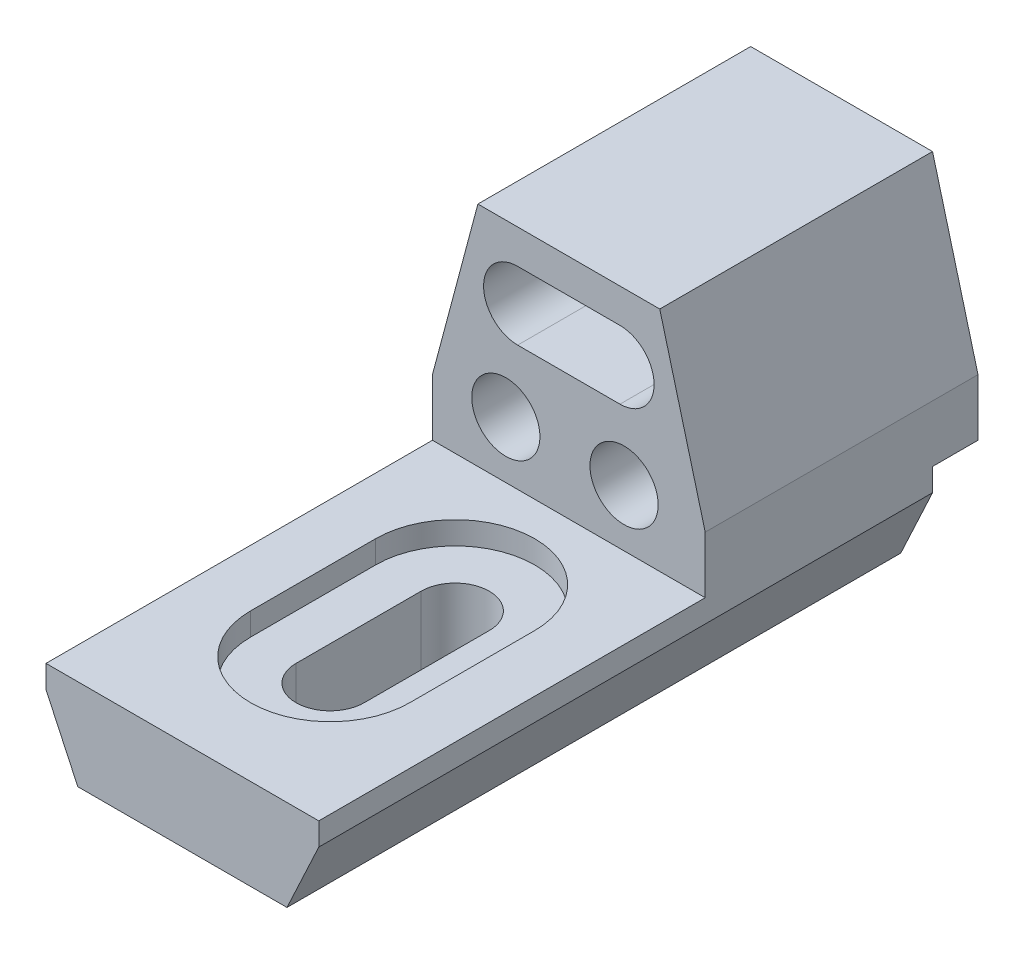
ISO-10303-21;
HEADER;
FILE_DESCRIPTION(('STEP AP214'),'2;1');
FILE_NAME('part.step','',(''),(''),'','','');
FILE_SCHEMA(('AUTOMOTIVE_DESIGN { 1 0 10303 214 1 1 1 1 }'));
ENDSEC;
DATA;
#1=APPLICATION_CONTEXT('core data for automotive mechanical design processes');
#2=APPLICATION_PROTOCOL_DEFINITION('international standard','automotive_design',2000,#1);
#3=PRODUCT_CONTEXT('',#1,'mechanical');
#4=PRODUCT('Part','Part','',(#3));
#5=PRODUCT_RELATED_PRODUCT_CATEGORY('part','',(#4));
#6=PRODUCT_DEFINITION_FORMATION('','',#4);
#7=PRODUCT_DEFINITION_CONTEXT('part definition',#1,'design');
#8=PRODUCT_DEFINITION('design','',#6,#7);
#9=PRODUCT_DEFINITION_SHAPE('','',#8);
#10=(LENGTH_UNIT() NAMED_UNIT(*) SI_UNIT(.MILLI.,.METRE.));
#11=(NAMED_UNIT(*) PLANE_ANGLE_UNIT() SI_UNIT($,.RADIAN.));
#12=(NAMED_UNIT(*) SI_UNIT($,.STERADIAN.) SOLID_ANGLE_UNIT());
#13=UNCERTAINTY_MEASURE_WITH_UNIT(LENGTH_MEASURE(1.E-05),#10,'distance_accuracy_value','');
#14=(GEOMETRIC_REPRESENTATION_CONTEXT(3) GLOBAL_UNCERTAINTY_ASSIGNED_CONTEXT((#13)) GLOBAL_UNIT_ASSIGNED_CONTEXT((#10,
#11,#12)) REPRESENTATION_CONTEXT('',''));
#15=CARTESIAN_POINT('',(0.,0.,0.));
#16=DIRECTION('',(0.,0.,1.));
#17=DIRECTION('',(1.,0.,0.));
#18=AXIS2_PLACEMENT_3D('',#15,#16,#17);
#19=CARTESIAN_POINT('',(0.,40.,-290.));
#20=DIRECTION('',(0.,-1.,0.));
#21=DIRECTION('',(0.,0.,-1.));
#22=AXIS2_PLACEMENT_3D('',#19,#20,#21);
#23=PLANE('',#22);
#24=DIRECTION('',(0.,0.,1.));
#25=VECTOR('',#24,1.);
#26=CARTESIAN_POINT('',(11.0107702553499,40.,-120.));
#27=LINE('',#26,#25);
#28=CARTESIAN_POINT('',(11.0107702553499,40.,-120.));
#29=VERTEX_POINT('',#28);
#30=CARTESIAN_POINT('',(11.0107702553498,40.,-65.));
#31=VERTEX_POINT('',#30);
#32=EDGE_CURVE('E349',#29,#31,#27,.T.);
#33=ORIENTED_EDGE('',*,*,#32,.F.);
#34=CARTESIAN_POINT('',(46.0107702553499,40.,-120.));
#35=DIRECTION('',(0.,1.,0.));
#36=DIRECTION('',(0.,0.,1.));
#37=AXIS2_PLACEMENT_3D('',#34,#35,#36);
#38=CIRCLE('',#37,35.);
#39=CARTESIAN_POINT('',(81.0107702553499,40.,-120.));
#40=VERTEX_POINT('',#39);
#41=EDGE_CURVE('E327',#40,#29,#38,.T.);
#42=ORIENTED_EDGE('',*,*,#41,.F.);
#43=DIRECTION('',(0.,0.,-1.));
#44=VECTOR('',#43,1.);
#45=CARTESIAN_POINT('',(81.0107702553499,40.,-120.));
#46=LINE('',#45,#44);
#47=CARTESIAN_POINT('',(81.0107702553499,40.,-65.));
#48=VERTEX_POINT('',#47);
#49=EDGE_CURVE('E340',#48,#40,#46,.T.);
#50=ORIENTED_EDGE('',*,*,#49,.F.);
#51=CARTESIAN_POINT('',(46.0107702553499,40.,-65.));
#52=DIRECTION('',(0.,1.,0.));
#53=DIRECTION('',(0.,0.,1.));
#54=AXIS2_PLACEMENT_3D('',#51,#52,#53);
#55=CIRCLE('',#54,35.);
#56=EDGE_CURVE('E353',#31,#48,#55,.T.);
#57=ORIENTED_EDGE('',*,*,#56,.F.);
#58=EDGE_LOOP('',(#33,#42,#50,#57));
#59=FACE_BOUND('',#58,.T.);
#60=DIRECTION('',(1.,0.,0.));
#61=VECTOR('',#60,1.);
#62=CARTESIAN_POINT('',(-13.9892297446501,40.,-170.));
#63=LINE('',#62,#61);
#64=CARTESIAN_POINT('',(-13.9892297446501,40.,-170.));
#65=VERTEX_POINT('',#64);
#66=CARTESIAN_POINT('',(106.01077025535,40.,-170.));
#67=VERTEX_POINT('',#66);
#68=EDGE_CURVE('E284',#65,#67,#63,.T.);
#69=ORIENTED_EDGE('',*,*,#68,.F.);
#70=DIRECTION('',(0.,0.,1.));
#71=VECTOR('',#70,1.);
#72=CARTESIAN_POINT('',(-13.9892297446501,40.,-290.));
#73=LINE('',#72,#71);
#74=CARTESIAN_POINT('',(-13.9892297446501,40.,0.));
#75=VERTEX_POINT('',#74);
#76=EDGE_CURVE('E395',#65,#75,#73,.T.);
#77=ORIENTED_EDGE('',*,*,#76,.T.);
#78=DIRECTION('',(1.,0.,0.));
#79=VECTOR('',#78,1.);
#80=CARTESIAN_POINT('',(0.,40.,0.));
#81=LINE('',#80,#79);
#82=CARTESIAN_POINT('',(106.01077025535,40.,0.));
#83=VERTEX_POINT('',#82);
#84=EDGE_CURVE('E370',#75,#83,#81,.T.);
#85=ORIENTED_EDGE('',*,*,#84,.T.);
#86=DIRECTION('',(0.,0.,1.));
#87=VECTOR('',#86,1.);
#88=CARTESIAN_POINT('',(106.01077025535,40.,-290.));
#89=LINE('',#88,#87);
#90=EDGE_CURVE('E385',#67,#83,#89,.T.);
#91=ORIENTED_EDGE('',*,*,#90,.F.);
#92=EDGE_LOOP('',(#69,#77,#85,#91));
#93=FACE_BOUND('',#92,.T.);
#94=ADVANCED_FACE('F50',(#59,#93),#23,.F.);
#95=CARTESIAN_POINT('',(106.01077025535,0.,-290.));
#96=DIRECTION('',(-1.,0.,0.));
#97=DIRECTION('',(0.,0.,1.));
#98=AXIS2_PLACEMENT_3D('',#95,#96,#97);
#99=PLANE('',#98);
#100=DIRECTION('',(0.,0.,1.));
#101=VECTOR('',#100,1.);
#102=CARTESIAN_POINT('',(106.01077025535,30.,-290.));
#103=LINE('',#102,#101);
#104=CARTESIAN_POINT('',(106.01077025535,30.,-270.));
#105=VERTEX_POINT('',#104);
#106=CARTESIAN_POINT('',(106.01077025535,30.,0.));
#107=VERTEX_POINT('',#106);
#108=EDGE_CURVE('E384',#105,#107,#103,.T.);
#109=ORIENTED_EDGE('',*,*,#108,.F.);
#110=DIRECTION('',(0.,1.,0.));
#111=VECTOR('',#110,1.);
#112=CARTESIAN_POINT('',(106.01077025535,-10.,-270.));
#113=LINE('',#112,#111);
#114=CARTESIAN_POINT('',(106.01077025535,40.,-270.));
#115=VERTEX_POINT('',#114);
#116=EDGE_CURVE('E301',#105,#115,#113,.T.);
#117=ORIENTED_EDGE('',*,*,#116,.T.);
#118=DIRECTION('',(0.,0.,-1.));
#119=VECTOR('',#118,1.);
#120=CARTESIAN_POINT('',(106.01077025535,40.,-170.));
#121=LINE('',#120,#119);
#122=CARTESIAN_POINT('',(106.01077025535,40.,-290.));
#123=VERTEX_POINT('',#122);
#124=EDGE_CURVE('E274',#115,#123,#121,.T.);
#125=ORIENTED_EDGE('',*,*,#124,.T.);
#126=DIRECTION('',(0.,-1.,0.));
#127=VECTOR('',#126,1.);
#128=CARTESIAN_POINT('',(106.01077025535,65.,-290.));
#129=LINE('',#128,#127);
#130=CARTESIAN_POINT('',(106.01077025535,65.,-290.));
#131=VERTEX_POINT('',#130);
#132=EDGE_CURVE('E280',#131,#123,#129,.T.);
#133=ORIENTED_EDGE('',*,*,#132,.F.);
#134=DIRECTION('',(0.,0.,-1.));
#135=VECTOR('',#134,1.);
#136=CARTESIAN_POINT('',(106.01077025535,65.,-170.));
#137=LINE('',#136,#135);
#138=CARTESIAN_POINT('',(106.01077025535,65.,-170.));
#139=VERTEX_POINT('',#138);
#140=EDGE_CURVE('E271',#139,#131,#137,.T.);
#141=ORIENTED_EDGE('',*,*,#140,.F.);
#142=DIRECTION('',(0.,-1.,0.));
#143=VECTOR('',#142,1.);
#144=CARTESIAN_POINT('',(106.01077025535,65.,-170.));
#145=LINE('',#144,#143);
#146=EDGE_CURVE('E289',#139,#67,#145,.T.);
#147=ORIENTED_EDGE('',*,*,#146,.T.);
#148=ORIENTED_EDGE('',*,*,#90,.T.);
#149=DIRECTION('',(0.,-1.,0.));
#150=VECTOR('',#149,1.);
#151=CARTESIAN_POINT('',(106.01077025535,0.,0.));
#152=LINE('',#151,#150);
#153=EDGE_CURVE('E356',#83,#107,#152,.T.);
#154=ORIENTED_EDGE('',*,*,#153,.T.);
#155=EDGE_LOOP('',(#109,#117,#125,#133,#141,#147,#148,#154));
#156=FACE_BOUND('',#155,.T.);
#157=ADVANCED_FACE('F47',(#156),#99,.F.);
#158=CARTESIAN_POINT('',(75.5859232876231,-35.2462948777347,-290.));
#159=DIRECTION('',(0.906307787036651,-0.422618261740697,0.));
#160=DIRECTION('',(0.422618261740697,0.906307787036651,0.));
#161=AXIS2_PLACEMENT_3D('',#158,#159,#160);
#162=PLANE('',#161);
#163=DIRECTION('',(-0.422618261740697,-0.906307787036651,0.));
#164=VECTOR('',#163,1.);
#165=CARTESIAN_POINT('',(75.5859232876231,-35.2462948777347,-270.));
#166=LINE('',#165,#164);
#167=CARTESIAN_POINT('',(92.0215405107,0.,-270.));
#168=VERTEX_POINT('',#167);
#169=EDGE_CURVE('E309',#105,#168,#166,.T.);
#170=ORIENTED_EDGE('',*,*,#169,.F.);
#171=ORIENTED_EDGE('',*,*,#108,.T.);
#172=DIRECTION('',(0.422618261740697,0.906307787036651,0.));
#173=VECTOR('',#172,1.);
#174=CARTESIAN_POINT('',(75.5859232876231,-35.2462948777347,0.));
#175=LINE('',#174,#173);
#176=CARTESIAN_POINT('',(92.0215405107,0.,0.));
#177=VERTEX_POINT('',#176);
#178=EDGE_CURVE('E378',#177,#107,#175,.T.);
#179=ORIENTED_EDGE('',*,*,#178,.F.);
#180=DIRECTION('',(0.,0.,1.));
#181=VECTOR('',#180,1.);
#182=CARTESIAN_POINT('',(92.0215405107,0.,-290.));
#183=LINE('',#182,#181);
#184=EDGE_CURVE('E387',#168,#177,#183,.T.);
#185=ORIENTED_EDGE('',*,*,#184,.F.);
#186=EDGE_LOOP('',(#170,#171,#179,#185));
#187=FACE_BOUND('',#186,.T.);
#188=ADVANCED_FACE('F521',(#187),#162,.T.);
#189=CARTESIAN_POINT('',(0.,0.,-290.));
#190=DIRECTION('',(0.,-1.,0.));
#191=DIRECTION('',(0.,0.,-1.));
#192=AXIS2_PLACEMENT_3D('',#189,#190,#191);
#193=PLANE('',#192);
#194=DIRECTION('',(-1.,0.,0.));
#195=VECTOR('',#194,1.);
#196=CARTESIAN_POINT('',(0.,0.,-270.));
#197=LINE('',#196,#195);
#198=CARTESIAN_POINT('',(0.,0.,-270.));
#199=VERTEX_POINT('',#198);
#200=EDGE_CURVE('E308',#168,#199,#197,.T.);
#201=ORIENTED_EDGE('',*,*,#200,.F.);
#202=ORIENTED_EDGE('',*,*,#184,.T.);
#203=DIRECTION('',(1.,0.,0.));
#204=VECTOR('',#203,1.);
#205=CARTESIAN_POINT('',(0.,0.,0.));
#206=LINE('',#205,#204);
#207=CARTESIAN_POINT('',(0.,0.,0.));
#208=VERTEX_POINT('',#207);
#209=EDGE_CURVE('E376',#208,#177,#206,.T.);
#210=ORIENTED_EDGE('',*,*,#209,.F.);
#211=DIRECTION('',(0.,0.,1.));
#212=VECTOR('',#211,1.);
#213=CARTESIAN_POINT('',(0.,0.,-290.));
#214=LINE('',#213,#212);
#215=EDGE_CURVE('E389',#199,#208,#214,.T.);
#216=ORIENTED_EDGE('',*,*,#215,.F.);
#217=EDGE_LOOP('',(#201,#202,#210,#216));
#218=FACE_BOUND('',#217,.T.);
#219=CARTESIAN_POINT('',(46.0107702553499,0.,-120.));
#220=DIRECTION('',(0.,-1.,0.));
#221=DIRECTION('',(0.,0.,-1.));
#222=AXIS2_PLACEMENT_3D('',#219,#220,#221);
#223=CIRCLE('',#222,15.);
#224=CARTESIAN_POINT('',(31.0107702553499,0.,-120.));
#225=VERTEX_POINT('',#224);
#226=CARTESIAN_POINT('',(61.0107702553499,0.,-120.));
#227=VERTEX_POINT('',#226);
#228=EDGE_CURVE('E11',#225,#227,#223,.T.);
#229=ORIENTED_EDGE('',*,*,#228,.F.);
#230=DIRECTION('',(0.,0.,-1.));
#231=VECTOR('',#230,1.);
#232=CARTESIAN_POINT('',(31.0107702553498,0.,-290.));
#233=LINE('',#232,#231);
#234=CARTESIAN_POINT('',(31.0107702553499,0.,-65.));
#235=VERTEX_POINT('',#234);
#236=EDGE_CURVE('E383',#235,#225,#233,.T.);
#237=ORIENTED_EDGE('',*,*,#236,.F.);
#238=CARTESIAN_POINT('',(46.0107702553499,0.,-65.));
#239=DIRECTION('',(0.,-1.,0.));
#240=DIRECTION('',(0.,0.,-1.));
#241=AXIS2_PLACEMENT_3D('',#238,#239,#240);
#242=CIRCLE('',#241,15.);
#243=CARTESIAN_POINT('',(61.0107702553499,0.,-65.));
#244=VERTEX_POINT('',#243);
#245=EDGE_CURVE('E398',#244,#235,#242,.T.);
#246=ORIENTED_EDGE('',*,*,#245,.F.);
#247=DIRECTION('',(0.,0.,1.));
#248=VECTOR('',#247,1.);
#249=CARTESIAN_POINT('',(61.0107702553499,0.,-290.));
#250=LINE('',#249,#248);
#251=EDGE_CURVE('E54',#227,#244,#250,.T.);
#252=ORIENTED_EDGE('',*,*,#251,.F.);
#253=EDGE_LOOP('',(#229,#237,#246,#252));
#254=FACE_BOUND('',#253,.T.);
#255=ADVANCED_FACE('F412',(#218,#254),#193,.T.);
#256=CARTESIAN_POINT('',(0.,0.,-290.));
#257=DIRECTION('',(0.906307787036648,0.422618261740704,0.));
#258=DIRECTION('',(-0.422618261740704,0.906307787036648,0.));
#259=AXIS2_PLACEMENT_3D('',#256,#257,#258);
#260=PLANE('',#259);
#261=DIRECTION('',(0.,0.,1.));
#262=VECTOR('',#261,1.);
#263=CARTESIAN_POINT('',(-13.9892297446501,30.,-290.));
#264=LINE('',#263,#262);
#265=CARTESIAN_POINT('',(-13.9892297446501,30.,-270.));
#266=VERTEX_POINT('',#265);
#267=CARTESIAN_POINT('',(-13.9892297446501,30.,0.));
#268=VERTEX_POINT('',#267);
#269=EDGE_CURVE('E388',#266,#268,#264,.T.);
#270=ORIENTED_EDGE('',*,*,#269,.F.);
#271=DIRECTION('',(0.422618261740704,-0.906307787036648,0.));
#272=VECTOR('',#271,1.);
#273=CARTESIAN_POINT('',(0.,0.,-270.));
#274=LINE('',#273,#272);
#275=EDGE_CURVE('E302',#266,#199,#274,.T.);
#276=ORIENTED_EDGE('',*,*,#275,.T.);
#277=ORIENTED_EDGE('',*,*,#215,.T.);
#278=DIRECTION('',(-0.422618261740704,0.906307787036648,0.));
#279=VECTOR('',#278,1.);
#280=CARTESIAN_POINT('',(0.,0.,0.));
#281=LINE('',#280,#279);
#282=EDGE_CURVE('E373',#208,#268,#281,.T.);
#283=ORIENTED_EDGE('',*,*,#282,.T.);
#284=EDGE_LOOP('',(#270,#276,#277,#283));
#285=FACE_BOUND('',#284,.T.);
#286=ADVANCED_FACE('F470',(#285),#260,.F.);
#287=CARTESIAN_POINT('',(-13.9892297446501,0.,-290.));
#288=DIRECTION('',(1.,0.,0.));
#289=DIRECTION('',(0.,0.,-1.));
#290=AXIS2_PLACEMENT_3D('',#287,#288,#289);
#291=PLANE('',#290);
#292=ORIENTED_EDGE('',*,*,#76,.F.);
#293=DIRECTION('',(0.,-1.,0.));
#294=VECTOR('',#293,1.);
#295=CARTESIAN_POINT('',(-13.9892297446501,65.,-170.));
#296=LINE('',#295,#294);
#297=CARTESIAN_POINT('',(-13.9892297446501,65.,-170.));
#298=VERTEX_POINT('',#297);
#299=EDGE_CURVE('E292',#298,#65,#296,.T.);
#300=ORIENTED_EDGE('',*,*,#299,.F.);
#301=DIRECTION('',(0.,0.,1.));
#302=VECTOR('',#301,1.);
#303=CARTESIAN_POINT('',(-13.9892297446501,65.,-290.));
#304=LINE('',#303,#302);
#305=CARTESIAN_POINT('',(-13.9892297446501,65.,-290.));
#306=VERTEX_POINT('',#305);
#307=EDGE_CURVE('E267',#306,#298,#304,.T.);
#308=ORIENTED_EDGE('',*,*,#307,.F.);
#309=DIRECTION('',(0.,-1.,0.));
#310=VECTOR('',#309,1.);
#311=CARTESIAN_POINT('',(-13.9892297446501,65.,-290.));
#312=LINE('',#311,#310);
#313=CARTESIAN_POINT('',(-13.9892297446501,40.,-290.));
#314=VERTEX_POINT('',#313);
#315=EDGE_CURVE('E294',#306,#314,#312,.T.);
#316=ORIENTED_EDGE('',*,*,#315,.T.);
#317=DIRECTION('',(0.,0.,1.));
#318=VECTOR('',#317,1.);
#319=CARTESIAN_POINT('',(-13.9892297446501,40.,-290.));
#320=LINE('',#319,#318);
#321=CARTESIAN_POINT('',(-13.9892297446501,40.,-270.));
#322=VERTEX_POINT('',#321);
#323=EDGE_CURVE('E278',#314,#322,#320,.T.);
#324=ORIENTED_EDGE('',*,*,#323,.T.);
#325=DIRECTION('',(0.,1.,0.));
#326=VECTOR('',#325,1.);
#327=CARTESIAN_POINT('',(-13.9892297446501,-10.,-270.));
#328=LINE('',#327,#326);
#329=EDGE_CURVE('E297',#266,#322,#328,.T.);
#330=ORIENTED_EDGE('',*,*,#329,.F.);
#331=ORIENTED_EDGE('',*,*,#269,.T.);
#332=DIRECTION('',(0.,1.,0.));
#333=VECTOR('',#332,1.);
#334=CARTESIAN_POINT('',(-13.9892297446501,0.,0.));
#335=LINE('',#334,#333);
#336=EDGE_CURVE('E369',#268,#75,#335,.T.);
#337=ORIENTED_EDGE('',*,*,#336,.T.);
#338=EDGE_LOOP('',(#292,#300,#308,#316,#324,#330,#331,#337));
#339=FACE_BOUND('',#338,.T.);
#340=ADVANCED_FACE('F447',(#339),#291,.F.);
#341=CARTESIAN_POINT('',(0.,0.,0.));
#342=DIRECTION('',(0.,0.,1.));
#343=DIRECTION('',(1.,0.,0.));
#344=AXIS2_PLACEMENT_3D('',#341,#342,#343);
#345=PLANE('',#344);
#346=ORIENTED_EDGE('',*,*,#153,.F.);
#347=ORIENTED_EDGE('',*,*,#84,.F.);
#348=ORIENTED_EDGE('',*,*,#336,.F.);
#349=ORIENTED_EDGE('',*,*,#282,.F.);
#350=ORIENTED_EDGE('',*,*,#209,.T.);
#351=ORIENTED_EDGE('',*,*,#178,.T.);
#352=EDGE_LOOP('',(#346,#347,#348,#349,#350,#351));
#353=FACE_BOUND('',#352,.T.);
#354=ADVANCED_FACE('F474',(#353),#345,.T.);
#355=CARTESIAN_POINT('',(46.0107702553499,30.,-120.));
#356=DIRECTION('',(0.,1.,0.));
#357=DIRECTION('',(0.,0.,1.));
#358=AXIS2_PLACEMENT_3D('',#355,#356,#357);
#359=CYLINDRICAL_SURFACE('',#358,35.);
#360=ORIENTED_EDGE('',*,*,#41,.T.);
#361=DIRECTION('',(0.,1.,0.));
#362=VECTOR('',#361,1.);
#363=CARTESIAN_POINT('',(11.0107702553499,30.,-120.));
#364=LINE('',#363,#362);
#365=CARTESIAN_POINT('',(11.0107702553499,30.,-120.));
#366=VERTEX_POINT('',#365);
#367=EDGE_CURVE('E347',#366,#29,#364,.T.);
#368=ORIENTED_EDGE('',*,*,#367,.F.);
#369=CARTESIAN_POINT('',(46.0107702553499,30.,-120.));
#370=DIRECTION('',(0.,1.,0.));
#371=DIRECTION('',(0.,0.,1.));
#372=AXIS2_PLACEMENT_3D('',#369,#370,#371);
#373=CIRCLE('',#372,35.);
#374=CARTESIAN_POINT('',(81.0107702553499,30.,-120.));
#375=VERTEX_POINT('',#374);
#376=EDGE_CURVE('E331',#375,#366,#373,.T.);
#377=ORIENTED_EDGE('',*,*,#376,.F.);
#378=DIRECTION('',(0.,1.,0.));
#379=VECTOR('',#378,1.);
#380=CARTESIAN_POINT('',(81.0107702553499,30.,-120.));
#381=LINE('',#380,#379);
#382=EDGE_CURVE('E358',#375,#40,#381,.T.);
#383=ORIENTED_EDGE('',*,*,#382,.T.);
#384=EDGE_LOOP('',(#360,#368,#377,#383));
#385=FACE_BOUND('',#384,.T.);
#386=ADVANCED_FACE('F429',(#385),#359,.F.);
#387=CARTESIAN_POINT('',(81.0107702553499,30.,-120.));
#388=DIRECTION('',(1.,0.,0.));
#389=DIRECTION('',(0.,0.,-1.));
#390=AXIS2_PLACEMENT_3D('',#387,#388,#389);
#391=PLANE('',#390);
#392=ORIENTED_EDGE('',*,*,#49,.T.);
#393=ORIENTED_EDGE('',*,*,#382,.F.);
#394=DIRECTION('',(0.,0.,-1.));
#395=VECTOR('',#394,1.);
#396=CARTESIAN_POINT('',(81.0107702553499,30.,-120.));
#397=LINE('',#396,#395);
#398=CARTESIAN_POINT('',(81.0107702553499,30.,-65.));
#399=VERTEX_POINT('',#398);
#400=EDGE_CURVE('E344',#399,#375,#397,.T.);
#401=ORIENTED_EDGE('',*,*,#400,.F.);
#402=DIRECTION('',(0.,1.,0.));
#403=VECTOR('',#402,1.);
#404=CARTESIAN_POINT('',(81.0107702553499,30.,-65.));
#405=LINE('',#404,#403);
#406=EDGE_CURVE('E360',#399,#48,#405,.T.);
#407=ORIENTED_EDGE('',*,*,#406,.T.);
#408=EDGE_LOOP('',(#392,#393,#401,#407));
#409=FACE_BOUND('',#408,.T.);
#410=ADVANCED_FACE('F438',(#409),#391,.F.);
#411=CARTESIAN_POINT('',(46.0107702553499,30.,-65.));
#412=DIRECTION('',(0.,1.,0.));
#413=DIRECTION('',(0.,0.,1.));
#414=AXIS2_PLACEMENT_3D('',#411,#412,#413);
#415=CYLINDRICAL_SURFACE('',#414,35.);
#416=ORIENTED_EDGE('',*,*,#56,.T.);
#417=ORIENTED_EDGE('',*,*,#406,.F.);
#418=CARTESIAN_POINT('',(46.0107702553499,30.,-65.));
#419=DIRECTION('',(0.,1.,0.));
#420=DIRECTION('',(0.,0.,1.));
#421=AXIS2_PLACEMENT_3D('',#418,#419,#420);
#422=CIRCLE('',#421,35.);
#423=CARTESIAN_POINT('',(11.0107702553498,30.,-65.));
#424=VERTEX_POINT('',#423);
#425=EDGE_CURVE('E338',#424,#399,#422,.T.);
#426=ORIENTED_EDGE('',*,*,#425,.F.);
#427=DIRECTION('',(0.,1.,0.));
#428=VECTOR('',#427,1.);
#429=CARTESIAN_POINT('',(11.0107702553498,30.,-65.));
#430=LINE('',#429,#428);
#431=EDGE_CURVE('E363',#424,#31,#430,.T.);
#432=ORIENTED_EDGE('',*,*,#431,.T.);
#433=EDGE_LOOP('',(#416,#417,#426,#432));
#434=FACE_BOUND('',#433,.T.);
#435=ADVANCED_FACE('F436',(#434),#415,.F.);
#436=CARTESIAN_POINT('',(11.0107702553499,30.,-120.));
#437=DIRECTION('',(-1.,0.,0.));
#438=DIRECTION('',(0.,0.,1.));
#439=AXIS2_PLACEMENT_3D('',#436,#437,#438);
#440=PLANE('',#439);
#441=ORIENTED_EDGE('',*,*,#32,.T.);
#442=ORIENTED_EDGE('',*,*,#431,.F.);
#443=DIRECTION('',(0.,0.,1.));
#444=VECTOR('',#443,1.);
#445=CARTESIAN_POINT('',(11.0107702553499,30.,-120.));
#446=LINE('',#445,#444);
#447=EDGE_CURVE('E337',#366,#424,#446,.T.);
#448=ORIENTED_EDGE('',*,*,#447,.F.);
#449=ORIENTED_EDGE('',*,*,#367,.T.);
#450=EDGE_LOOP('',(#441,#442,#448,#449));
#451=FACE_BOUND('',#450,.T.);
#452=ADVANCED_FACE('F421',(#451),#440,.F.);
#453=CARTESIAN_POINT('',(46.0107702553499,30.,-120.));
#454=DIRECTION('',(0.,1.,0.));
#455=DIRECTION('',(0.,0.,1.));
#456=AXIS2_PLACEMENT_3D('',#453,#454,#455);
#457=PLANE('',#456);
#458=CARTESIAN_POINT('',(46.0107702553499,30.,-120.));
#459=DIRECTION('',(0.,1.,0.));
#460=DIRECTION('',(0.,0.,1.));
#461=AXIS2_PLACEMENT_3D('',#458,#459,#460);
#462=CIRCLE('',#461,15.);
#463=CARTESIAN_POINT('',(61.0107702553499,30.,-120.));
#464=VERTEX_POINT('',#463);
#465=CARTESIAN_POINT('',(31.0107702553499,30.,-120.));
#466=VERTEX_POINT('',#465);
#467=EDGE_CURVE('E315',#464,#466,#462,.T.);
#468=ORIENTED_EDGE('',*,*,#467,.F.);
#469=DIRECTION('',(0.,0.,-1.));
#470=VECTOR('',#469,1.);
#471=CARTESIAN_POINT('',(61.0107702553499,30.,-120.));
#472=LINE('',#471,#470);
#473=CARTESIAN_POINT('',(61.0107702553499,30.,-65.));
#474=VERTEX_POINT('',#473);
#475=EDGE_CURVE('E318',#474,#464,#472,.T.);
#476=ORIENTED_EDGE('',*,*,#475,.F.);
#477=CARTESIAN_POINT('',(46.0107702553499,30.,-65.));
#478=DIRECTION('',(0.,1.,0.));
#479=DIRECTION('',(0.,0.,1.));
#480=AXIS2_PLACEMENT_3D('',#477,#478,#479);
#481=CIRCLE('',#480,15.);
#482=CARTESIAN_POINT('',(31.0107702553499,30.,-65.));
#483=VERTEX_POINT('',#482);
#484=EDGE_CURVE('E319',#483,#474,#481,.T.);
#485=ORIENTED_EDGE('',*,*,#484,.F.);
#486=DIRECTION('',(0.,0.,1.));
#487=VECTOR('',#486,1.);
#488=CARTESIAN_POINT('',(31.0107702553499,30.,-120.));
#489=LINE('',#488,#487);
#490=EDGE_CURVE('E314',#466,#483,#489,.T.);
#491=ORIENTED_EDGE('',*,*,#490,.F.);
#492=EDGE_LOOP('',(#468,#476,#485,#491));
#493=FACE_BOUND('',#492,.T.);
#494=ORIENTED_EDGE('',*,*,#376,.T.);
#495=ORIENTED_EDGE('',*,*,#447,.T.);
#496=ORIENTED_EDGE('',*,*,#425,.T.);
#497=ORIENTED_EDGE('',*,*,#400,.T.);
#498=EDGE_LOOP('',(#494,#495,#496,#497));
#499=FACE_BOUND('',#498,.T.);
#500=ADVANCED_FACE('F417',(#493,#499),#457,.T.);
#501=CARTESIAN_POINT('',(46.0107702553499,-20.,-120.));
#502=DIRECTION('',(0.,1.,0.));
#503=DIRECTION('',(0.,0.,1.));
#504=AXIS2_PLACEMENT_3D('',#501,#502,#503);
#505=CYLINDRICAL_SURFACE('',#504,15.);
#506=ORIENTED_EDGE('',*,*,#228,.T.);
#507=DIRECTION('',(0.,1.,0.));
#508=VECTOR('',#507,1.);
#509=CARTESIAN_POINT('',(61.0107702553499,-20.,-120.));
#510=LINE('',#509,#508);
#511=EDGE_CURVE('E321',#227,#464,#510,.T.);
#512=ORIENTED_EDGE('',*,*,#511,.T.);
#513=ORIENTED_EDGE('',*,*,#467,.T.);
#514=DIRECTION('',(0.,1.,0.));
#515=VECTOR('',#514,1.);
#516=CARTESIAN_POINT('',(31.0107702553499,-20.,-120.));
#517=LINE('',#516,#515);
#518=EDGE_CURVE('E324',#225,#466,#517,.T.);
#519=ORIENTED_EDGE('',*,*,#518,.F.);
#520=EDGE_LOOP('',(#506,#512,#513,#519));
#521=FACE_BOUND('',#520,.T.);
#522=ADVANCED_FACE('F418',(#521),#505,.F.);
#523=CARTESIAN_POINT('',(61.0107702553499,-20.,-120.));
#524=DIRECTION('',(1.,0.,0.));
#525=DIRECTION('',(0.,0.,-1.));
#526=AXIS2_PLACEMENT_3D('',#523,#524,#525);
#527=PLANE('',#526);
#528=ORIENTED_EDGE('',*,*,#251,.T.);
#529=DIRECTION('',(0.,1.,0.));
#530=VECTOR('',#529,1.);
#531=CARTESIAN_POINT('',(61.0107702553499,-20.,-65.));
#532=LINE('',#531,#530);
#533=EDGE_CURVE('E330',#244,#474,#532,.T.);
#534=ORIENTED_EDGE('',*,*,#533,.T.);
#535=ORIENTED_EDGE('',*,*,#475,.T.);
#536=ORIENTED_EDGE('',*,*,#511,.F.);
#537=EDGE_LOOP('',(#528,#534,#535,#536));
#538=FACE_BOUND('',#537,.T.);
#539=ADVANCED_FACE('F405',(#538),#527,.F.);
#540=CARTESIAN_POINT('',(46.0107702553499,-20.,-65.));
#541=DIRECTION('',(0.,1.,0.));
#542=DIRECTION('',(0.,0.,1.));
#543=AXIS2_PLACEMENT_3D('',#540,#541,#542);
#544=CYLINDRICAL_SURFACE('',#543,15.);
#545=ORIENTED_EDGE('',*,*,#245,.T.);
#546=DIRECTION('',(0.,1.,0.));
#547=VECTOR('',#546,1.);
#548=CARTESIAN_POINT('',(31.0107702553499,-20.,-65.));
#549=LINE('',#548,#547);
#550=EDGE_CURVE('E328',#235,#483,#549,.T.);
#551=ORIENTED_EDGE('',*,*,#550,.T.);
#552=ORIENTED_EDGE('',*,*,#484,.T.);
#553=ORIENTED_EDGE('',*,*,#533,.F.);
#554=EDGE_LOOP('',(#545,#551,#552,#553));
#555=FACE_BOUND('',#554,.T.);
#556=ADVANCED_FACE('F409',(#555),#544,.F.);
#557=CARTESIAN_POINT('',(31.0107702553499,-20.,-120.));
#558=DIRECTION('',(-1.,0.,0.));
#559=DIRECTION('',(0.,0.,1.));
#560=AXIS2_PLACEMENT_3D('',#557,#558,#559);
#561=PLANE('',#560);
#562=ORIENTED_EDGE('',*,*,#236,.T.);
#563=ORIENTED_EDGE('',*,*,#518,.T.);
#564=ORIENTED_EDGE('',*,*,#490,.T.);
#565=ORIENTED_EDGE('',*,*,#550,.F.);
#566=EDGE_LOOP('',(#562,#563,#564,#565));
#567=FACE_BOUND('',#566,.T.);
#568=ADVANCED_FACE('F411',(#567),#561,.F.);
#569=CARTESIAN_POINT('',(106.01077025535,-10.,-270.));
#570=DIRECTION('',(0.,0.,1.));
#571=DIRECTION('',(1.,0.,0.));
#572=AXIS2_PLACEMENT_3D('',#569,#570,#571);
#573=PLANE('',#572);
#574=ORIENTED_EDGE('',*,*,#169,.T.);
#575=ORIENTED_EDGE('',*,*,#200,.T.);
#576=ORIENTED_EDGE('',*,*,#275,.F.);
#577=ORIENTED_EDGE('',*,*,#329,.T.);
#578=DIRECTION('',(1.,0.,0.));
#579=VECTOR('',#578,1.);
#580=CARTESIAN_POINT('',(106.01077025535,40.,-270.));
#581=LINE('',#580,#579);
#582=EDGE_CURVE('E296',#322,#115,#581,.T.);
#583=ORIENTED_EDGE('',*,*,#582,.T.);
#584=ORIENTED_EDGE('',*,*,#116,.F.);
#585=EDGE_LOOP('',(#574,#575,#576,#577,#583,#584));
#586=FACE_BOUND('',#585,.T.);
#587=ADVANCED_FACE('F505',(#586),#573,.F.);
#588=CARTESIAN_POINT('',(106.01077025535,65.,-290.));
#589=DIRECTION('',(0.,0.,1.));
#590=DIRECTION('',(1.,0.,0.));
#591=AXIS2_PLACEMENT_3D('',#588,#589,#590);
#592=PLANE('',#591);
#593=CARTESIAN_POINT('',(18.2996179978366,65.,-290.));
#594=DIRECTION('',(0.,0.,1.));
#595=DIRECTION('',(1.,0.,0.));
#596=AXIS2_PLACEMENT_3D('',#593,#594,#595);
#597=CIRCLE('',#596,15.);
#598=CARTESIAN_POINT('',(33.2996179978366,65.,-290.));
#599=VERTEX_POINT('',#598);
#600=EDGE_CURVE('E238',#599,#599,#597,.T.);
#601=ORIENTED_EDGE('',*,*,#600,.T.);
#602=EDGE_LOOP('',(#601));
#603=FACE_BOUND('',#602,.T.);
#604=CARTESIAN_POINT('',(70.2996179978366,65.,-290.));
#605=DIRECTION('',(0.,0.,1.));
#606=DIRECTION('',(1.,0.,0.));
#607=AXIS2_PLACEMENT_3D('',#604,#605,#606);
#608=CIRCLE('',#607,15.);
#609=CARTESIAN_POINT('',(85.2996179978366,65.,-290.));
#610=VERTEX_POINT('',#609);
#611=EDGE_CURVE('E814',#610,#610,#608,.T.);
#612=ORIENTED_EDGE('',*,*,#611,.T.);
#613=EDGE_LOOP('',(#612));
#614=FACE_BOUND('',#613,.T.);
#615=DIRECTION('',(-1.,0.,0.));
#616=VECTOR('',#615,1.);
#617=CARTESIAN_POINT('',(23.5107702553499,125.,-290.));
#618=LINE('',#617,#616);
#619=CARTESIAN_POINT('',(68.5107702553499,125.,-290.));
#620=VERTEX_POINT('',#619);
#621=CARTESIAN_POINT('',(23.5107702553499,125.,-290.));
#622=VERTEX_POINT('',#621);
#623=EDGE_CURVE('E213',#620,#622,#618,.T.);
#624=ORIENTED_EDGE('',*,*,#623,.T.);
#625=CARTESIAN_POINT('',(23.5107702553499,110.,-290.));
#626=DIRECTION('',(0.,0.,1.));
#627=DIRECTION('',(1.,0.,0.));
#628=AXIS2_PLACEMENT_3D('',#625,#626,#627);
#629=CIRCLE('',#628,15.);
#630=CARTESIAN_POINT('',(23.5107702553499,95.,-290.));
#631=VERTEX_POINT('',#630);
#632=EDGE_CURVE('E209',#622,#631,#629,.T.);
#633=ORIENTED_EDGE('',*,*,#632,.T.);
#634=DIRECTION('',(1.,0.,0.));
#635=VECTOR('',#634,1.);
#636=CARTESIAN_POINT('',(23.5107702553499,95.,-290.));
#637=LINE('',#636,#635);
#638=CARTESIAN_POINT('',(68.5107702553499,95.,-290.));
#639=VERTEX_POINT('',#638);
#640=EDGE_CURVE('E219',#631,#639,#637,.T.);
#641=ORIENTED_EDGE('',*,*,#640,.T.);
#642=CARTESIAN_POINT('',(68.5107702553499,110.,-290.));
#643=DIRECTION('',(0.,0.,1.));
#644=DIRECTION('',(1.,0.,0.));
#645=AXIS2_PLACEMENT_3D('',#642,#643,#644);
#646=CIRCLE('',#645,15.);
#647=EDGE_CURVE('E65',#639,#620,#646,.T.);
#648=ORIENTED_EDGE('',*,*,#647,.T.);
#649=EDGE_LOOP('',(#624,#633,#641,#648));
#650=FACE_BOUND('',#649,.T.);
#651=DIRECTION('',(-1.,0.,0.));
#652=VECTOR('',#651,1.);
#653=CARTESIAN_POINT('',(106.01077025535,40.,-290.));
#654=LINE('',#653,#652);
#655=EDGE_CURVE('E266',#123,#314,#654,.T.);
#656=ORIENTED_EDGE('',*,*,#655,.T.);
#657=ORIENTED_EDGE('',*,*,#315,.F.);
#658=DIRECTION('',(-0.257662650560332,-0.966234939601246,0.));
#659=VECTOR('',#658,1.);
#660=CARTESIAN_POINT('',(6.01077025534986,140.,-290.));
#661=LINE('',#660,#659);
#662=CARTESIAN_POINT('',(6.01077025534986,140.,-290.));
#663=VERTEX_POINT('',#662);
#664=EDGE_CURVE('E249',#663,#306,#661,.T.);
#665=ORIENTED_EDGE('',*,*,#664,.F.);
#666=DIRECTION('',(-1.,0.,0.));
#667=VECTOR('',#666,1.);
#668=CARTESIAN_POINT('',(46.0107702553499,140.,-290.));
#669=LINE('',#668,#667);
#670=CARTESIAN_POINT('',(86.0107702553499,140.,-290.));
#671=VERTEX_POINT('',#670);
#672=EDGE_CURVE('E247',#671,#663,#669,.T.);
#673=ORIENTED_EDGE('',*,*,#672,.F.);
#674=DIRECTION('',(-0.257662650560332,0.966234939601246,0.));
#675=VECTOR('',#674,1.);
#676=CARTESIAN_POINT('',(86.0107702553499,140.,-290.));
#677=LINE('',#676,#675);
#678=EDGE_CURVE('E251',#131,#671,#677,.T.);
#679=ORIENTED_EDGE('',*,*,#678,.F.);
#680=ORIENTED_EDGE('',*,*,#132,.T.);
#681=EDGE_LOOP('',(#656,#657,#665,#673,#679,#680));
#682=FACE_BOUND('',#681,.T.);
#683=ADVANCED_FACE('F225',(#603,#614,#650,#682),#592,.F.);
#684=CARTESIAN_POINT('',(-13.9892297446501,65.,-170.));
#685=DIRECTION('',(0.,0.,-1.));
#686=DIRECTION('',(-1.,0.,0.));
#687=AXIS2_PLACEMENT_3D('',#684,#685,#686);
#688=PLANE('',#687);
#689=CARTESIAN_POINT('',(18.2996179978366,65.,-170.));
#690=DIRECTION('',(0.,0.,1.));
#691=DIRECTION('',(1.,0.,0.));
#692=AXIS2_PLACEMENT_3D('',#689,#690,#691);
#693=CIRCLE('',#692,15.);
#694=CARTESIAN_POINT('',(33.2996179978366,65.,-170.));
#695=VERTEX_POINT('',#694);
#696=EDGE_CURVE('E815',#695,#695,#693,.T.);
#697=ORIENTED_EDGE('',*,*,#696,.F.);
#698=EDGE_LOOP('',(#697));
#699=FACE_BOUND('',#698,.T.);
#700=CARTESIAN_POINT('',(70.2996179978366,65.,-170.));
#701=DIRECTION('',(0.,0.,1.));
#702=DIRECTION('',(1.,0.,0.));
#703=AXIS2_PLACEMENT_3D('',#700,#701,#702);
#704=CIRCLE('',#703,15.);
#705=CARTESIAN_POINT('',(85.2996179978366,65.,-170.));
#706=VERTEX_POINT('',#705);
#707=EDGE_CURVE('E233',#706,#706,#704,.T.);
#708=ORIENTED_EDGE('',*,*,#707,.F.);
#709=EDGE_LOOP('',(#708));
#710=FACE_BOUND('',#709,.T.);
#711=DIRECTION('',(1.,0.,0.));
#712=VECTOR('',#711,1.);
#713=CARTESIAN_POINT('',(23.5107702553499,95.,-170.));
#714=LINE('',#713,#712);
#715=CARTESIAN_POINT('',(23.5107702553499,95.,-170.));
#716=VERTEX_POINT('',#715);
#717=CARTESIAN_POINT('',(68.5107702553499,95.,-170.));
#718=VERTEX_POINT('',#717);
#719=EDGE_CURVE('E240',#716,#718,#714,.T.);
#720=ORIENTED_EDGE('',*,*,#719,.F.);
#721=CARTESIAN_POINT('',(23.5107702553499,110.,-170.));
#722=DIRECTION('',(0.,0.,1.));
#723=DIRECTION('',(1.,0.,0.));
#724=AXIS2_PLACEMENT_3D('',#721,#722,#723);
#725=CIRCLE('',#724,15.);
#726=CARTESIAN_POINT('',(23.5107702553499,125.,-170.));
#727=VERTEX_POINT('',#726);
#728=EDGE_CURVE('E68',#727,#716,#725,.T.);
#729=ORIENTED_EDGE('',*,*,#728,.F.);
#730=DIRECTION('',(-1.,0.,0.));
#731=VECTOR('',#730,1.);
#732=CARTESIAN_POINT('',(23.5107702553499,125.,-170.));
#733=LINE('',#732,#731);
#734=CARTESIAN_POINT('',(68.5107702553499,125.,-170.));
#735=VERTEX_POINT('',#734);
#736=EDGE_CURVE('E222',#735,#727,#733,.T.);
#737=ORIENTED_EDGE('',*,*,#736,.F.);
#738=CARTESIAN_POINT('',(68.5107702553499,110.,-170.));
#739=DIRECTION('',(0.,0.,1.));
#740=DIRECTION('',(1.,0.,0.));
#741=AXIS2_PLACEMENT_3D('',#738,#739,#740);
#742=CIRCLE('',#741,15.);
#743=EDGE_CURVE('E226',#718,#735,#742,.T.);
#744=ORIENTED_EDGE('',*,*,#743,.F.);
#745=EDGE_LOOP('',(#720,#729,#737,#744));
#746=FACE_BOUND('',#745,.T.);
#747=ORIENTED_EDGE('',*,*,#68,.T.);
#748=ORIENTED_EDGE('',*,*,#146,.F.);
#749=DIRECTION('',(-0.257662650560332,0.966234939601246,0.));
#750=VECTOR('',#749,1.);
#751=CARTESIAN_POINT('',(86.0107702553499,140.,-170.));
#752=LINE('',#751,#750);
#753=CARTESIAN_POINT('',(86.0107702553499,140.,-170.));
#754=VERTEX_POINT('',#753);
#755=EDGE_CURVE('E252',#139,#754,#752,.T.);
#756=ORIENTED_EDGE('',*,*,#755,.T.);
#757=DIRECTION('',(-1.,0.,0.));
#758=VECTOR('',#757,1.);
#759=CARTESIAN_POINT('',(46.0107702553499,140.,-170.));
#760=LINE('',#759,#758);
#761=CARTESIAN_POINT('',(6.01077025534986,140.,-170.));
#762=VERTEX_POINT('',#761);
#763=EDGE_CURVE('E242',#754,#762,#760,.T.);
#764=ORIENTED_EDGE('',*,*,#763,.T.);
#765=DIRECTION('',(-0.257662650560332,-0.966234939601246,0.));
#766=VECTOR('',#765,1.);
#767=CARTESIAN_POINT('',(6.01077025534986,140.,-170.));
#768=LINE('',#767,#766);
#769=EDGE_CURVE('E258',#762,#298,#768,.T.);
#770=ORIENTED_EDGE('',*,*,#769,.T.);
#771=ORIENTED_EDGE('',*,*,#299,.T.);
#772=EDGE_LOOP('',(#747,#748,#756,#764,#770,#771));
#773=FACE_BOUND('',#772,.T.);
#774=ADVANCED_FACE('F446',(#699,#710,#746,#773),#688,.F.);
#775=CARTESIAN_POINT('',(0.,40.,0.));
#776=DIRECTION('',(0.,1.,0.));
#777=DIRECTION('',(0.,0.,1.));
#778=AXIS2_PLACEMENT_3D('',#775,#776,#777);
#779=PLANE('',#778);
#780=ORIENTED_EDGE('',*,*,#582,.F.);
#781=ORIENTED_EDGE('',*,*,#323,.F.);
#782=ORIENTED_EDGE('',*,*,#655,.F.);
#783=ORIENTED_EDGE('',*,*,#124,.F.);
#784=EDGE_LOOP('',(#780,#781,#782,#783));
#785=FACE_BOUND('',#784,.T.);
#786=ADVANCED_FACE('F465',(#785),#779,.F.);
#787=CARTESIAN_POINT('',(86.0107702553499,140.,-290.));
#788=DIRECTION('',(0.966234939601246,0.257662650560332,0.));
#789=DIRECTION('',(-0.257662650560332,0.966234939601247,0.));
#790=AXIS2_PLACEMENT_3D('',#787,#788,#789);
#791=PLANE('',#790);
#792=ORIENTED_EDGE('',*,*,#755,.F.);
#793=ORIENTED_EDGE('',*,*,#140,.T.);
#794=ORIENTED_EDGE('',*,*,#678,.T.);
#795=DIRECTION('',(0.,0.,1.));
#796=VECTOR('',#795,1.);
#797=CARTESIAN_POINT('',(86.0107702553499,140.,-290.));
#798=LINE('',#797,#796);
#799=EDGE_CURVE('E263',#671,#754,#798,.T.);
#800=ORIENTED_EDGE('',*,*,#799,.T.);
#801=EDGE_LOOP('',(#792,#793,#794,#800));
#802=FACE_BOUND('',#801,.T.);
#803=ADVANCED_FACE('F478',(#802),#791,.T.);
#804=CARTESIAN_POINT('',(6.01077025534986,140.,-290.));
#805=DIRECTION('',(-0.966234939601246,0.257662650560332,0.));
#806=DIRECTION('',(-0.257662650560332,-0.966234939601246,0.));
#807=AXIS2_PLACEMENT_3D('',#804,#805,#806);
#808=PLANE('',#807);
#809=ORIENTED_EDGE('',*,*,#769,.F.);
#810=DIRECTION('',(0.,0.,1.));
#811=VECTOR('',#810,1.);
#812=CARTESIAN_POINT('',(6.01077025534986,140.,-290.));
#813=LINE('',#812,#811);
#814=EDGE_CURVE('E260',#663,#762,#813,.T.);
#815=ORIENTED_EDGE('',*,*,#814,.F.);
#816=ORIENTED_EDGE('',*,*,#664,.T.);
#817=ORIENTED_EDGE('',*,*,#307,.T.);
#818=EDGE_LOOP('',(#809,#815,#816,#817));
#819=FACE_BOUND('',#818,.T.);
#820=ADVANCED_FACE('F454',(#819),#808,.T.);
#821=CARTESIAN_POINT('',(46.0107702553499,140.,-290.));
#822=DIRECTION('',(0.,1.,0.));
#823=DIRECTION('',(0.,0.,1.));
#824=AXIS2_PLACEMENT_3D('',#821,#822,#823);
#825=PLANE('',#824);
#826=ORIENTED_EDGE('',*,*,#763,.F.);
#827=ORIENTED_EDGE('',*,*,#799,.F.);
#828=ORIENTED_EDGE('',*,*,#672,.T.);
#829=ORIENTED_EDGE('',*,*,#814,.T.);
#830=EDGE_LOOP('',(#826,#827,#828,#829));
#831=FACE_BOUND('',#830,.T.);
#832=ADVANCED_FACE('F485',(#831),#825,.T.);
#833=CARTESIAN_POINT('',(23.5107702553499,110.,-290.));
#834=DIRECTION('',(0.,0.,1.));
#835=DIRECTION('',(1.,0.,0.));
#836=AXIS2_PLACEMENT_3D('',#833,#834,#835);
#837=CYLINDRICAL_SURFACE('',#836,15.);
#838=ORIENTED_EDGE('',*,*,#728,.T.);
#839=DIRECTION('',(0.,0.,1.));
#840=VECTOR('',#839,1.);
#841=CARTESIAN_POINT('',(23.5107702553499,95.,-290.));
#842=LINE('',#841,#840);
#843=EDGE_CURVE('E202',#631,#716,#842,.T.);
#844=ORIENTED_EDGE('',*,*,#843,.F.);
#845=ORIENTED_EDGE('',*,*,#632,.F.);
#846=DIRECTION('',(0.,0.,1.));
#847=VECTOR('',#846,1.);
#848=CARTESIAN_POINT('',(23.5107702553499,125.,-290.));
#849=LINE('',#848,#847);
#850=EDGE_CURVE('E245',#622,#727,#849,.T.);
#851=ORIENTED_EDGE('',*,*,#850,.T.);
#852=EDGE_LOOP('',(#838,#844,#845,#851));
#853=FACE_BOUND('',#852,.T.);
#854=ADVANCED_FACE('F210',(#853),#837,.F.);
#855=CARTESIAN_POINT('',(23.5107702553499,125.,-290.));
#856=DIRECTION('',(0.,1.,0.));
#857=DIRECTION('',(-1.,0.,0.));
#858=AXIS2_PLACEMENT_3D('',#855,#856,#857);
#859=PLANE('',#858);
#860=ORIENTED_EDGE('',*,*,#736,.T.);
#861=ORIENTED_EDGE('',*,*,#850,.F.);
#862=ORIENTED_EDGE('',*,*,#623,.F.);
#863=DIRECTION('',(0.,0.,1.));
#864=VECTOR('',#863,1.);
#865=CARTESIAN_POINT('',(68.5107702553499,125.,-290.));
#866=LINE('',#865,#864);
#867=EDGE_CURVE('E244',#620,#735,#866,.T.);
#868=ORIENTED_EDGE('',*,*,#867,.T.);
#869=EDGE_LOOP('',(#860,#861,#862,#868));
#870=FACE_BOUND('',#869,.T.);
#871=ADVANCED_FACE('F489',(#870),#859,.F.);
#872=CARTESIAN_POINT('',(68.5107702553499,110.,-290.));
#873=DIRECTION('',(0.,0.,1.));
#874=DIRECTION('',(1.,0.,0.));
#875=AXIS2_PLACEMENT_3D('',#872,#873,#874);
#876=CYLINDRICAL_SURFACE('',#875,15.);
#877=ORIENTED_EDGE('',*,*,#743,.T.);
#878=ORIENTED_EDGE('',*,*,#867,.F.);
#879=ORIENTED_EDGE('',*,*,#647,.F.);
#880=DIRECTION('',(0.,0.,1.));
#881=VECTOR('',#880,1.);
#882=CARTESIAN_POINT('',(68.5107702553499,95.,-290.));
#883=LINE('',#882,#881);
#884=EDGE_CURVE('E211',#639,#718,#883,.T.);
#885=ORIENTED_EDGE('',*,*,#884,.T.);
#886=EDGE_LOOP('',(#877,#878,#879,#885));
#887=FACE_BOUND('',#886,.T.);
#888=ADVANCED_FACE('F580',(#887),#876,.F.);
#889=CARTESIAN_POINT('',(23.5107702553499,95.,-290.));
#890=DIRECTION('',(0.,-1.,0.));
#891=DIRECTION('',(1.,0.,0.));
#892=AXIS2_PLACEMENT_3D('',#889,#890,#891);
#893=PLANE('',#892);
#894=ORIENTED_EDGE('',*,*,#719,.T.);
#895=ORIENTED_EDGE('',*,*,#884,.F.);
#896=ORIENTED_EDGE('',*,*,#640,.F.);
#897=ORIENTED_EDGE('',*,*,#843,.T.);
#898=EDGE_LOOP('',(#894,#895,#896,#897));
#899=FACE_BOUND('',#898,.T.);
#900=ADVANCED_FACE('F216',(#899),#893,.F.);
#901=CARTESIAN_POINT('',(70.2996179978366,65.,-290.));
#902=DIRECTION('',(0.,0.,1.));
#903=DIRECTION('',(1.,0.,0.));
#904=AXIS2_PLACEMENT_3D('',#901,#902,#903);
#905=CYLINDRICAL_SURFACE('',#904,15.);
#906=ORIENTED_EDGE('',*,*,#611,.F.);
#907=EDGE_LOOP('',(#906));
#908=FACE_BOUND('',#907,.T.);
#909=ORIENTED_EDGE('',*,*,#707,.T.);
#910=EDGE_LOOP('',(#909));
#911=FACE_BOUND('',#910,.T.);
#912=ADVANCED_FACE('F599',(#908,#911),#905,.F.);
#913=CARTESIAN_POINT('',(18.2996179978366,65.,-290.));
#914=DIRECTION('',(0.,0.,1.));
#915=DIRECTION('',(1.,0.,0.));
#916=AXIS2_PLACEMENT_3D('',#913,#914,#915);
#917=CYLINDRICAL_SURFACE('',#916,15.);
#918=ORIENTED_EDGE('',*,*,#600,.F.);
#919=EDGE_LOOP('',(#918));
#920=FACE_BOUND('',#919,.T.);
#921=ORIENTED_EDGE('',*,*,#696,.T.);
#922=EDGE_LOOP('',(#921));
#923=FACE_BOUND('',#922,.T.);
#924=ADVANCED_FACE('F608',(#920,#923),#917,.F.);
#925=CLOSED_SHELL('',(#94,#157,#188,#255,#286,#340,#354,#386,#410,#435,#452,#500,#522,#539,#556,
#568,#587,#683,#774,#786,#803,#820,#832,#854,#871,#888,#900,#912,#924));
#926=MANIFOLD_SOLID_BREP('B2',#925);
#927=ADVANCED_BREP_SHAPE_REPRESENTATION('',(#18,#926),#14);
#928=SHAPE_DEFINITION_REPRESENTATION(#9,#927);
ENDSEC;
END-ISO-10303-21;
